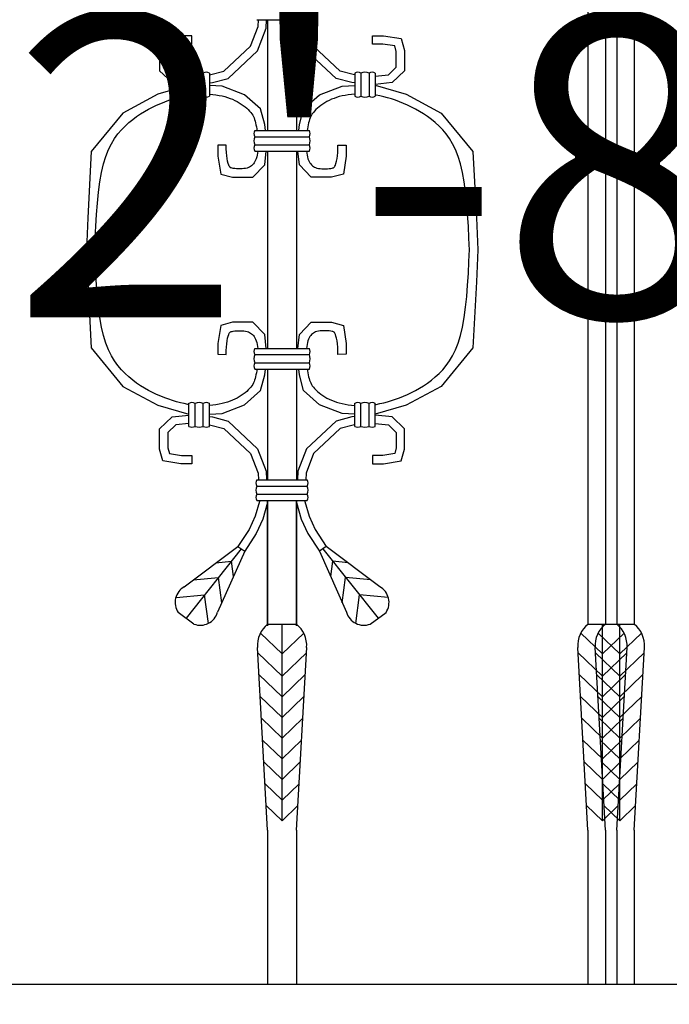
# Model space of a CAD drawing. Units: inches. Extents: x 2278 to 7495, y -71 to 1198.
# Tile 28 of 44: x 5114.19 to 5127.04, y 126.41 to 145.88. Entities that reach past the tile are written whole.
import ezdxf

# ---------------------------------------------------------------- set-up
doc = ezdxf.new("R2010")
doc.units = ezdxf.units.IN
doc.header["$MEASUREMENT"] = 0
doc.layers.add('A-ANNO-DIMS', color=2, linetype='Continuous', lineweight=18)
doc.layers.add('A-ELEV', color=7, linetype='Continuous', lineweight=25)
doc.styles.get("Standard").update_dxf_attribs({"font": 'arial.ttf'})
doc.dimstyles.get("Standard").update_dxf_attribs({"dimtxt": 6, "dimasz": 3, "dimexe": 0.18, "dimexo": 0.0625, "dimgap": 0.09, "dimtad": 0, "dimtih": 1, "dimtoh": 1, "dimdec": 0, "dimzin": 0, "dimdsep": 46, "dimlunit": 3, "dimtxsty": 'Standard', "dimblk": 'ARCHTICK', "dimcen": 0.09, "dimadec": 0, "dimazin": 0, "dimtfac": 1, "dimtdec": 0, "dimtofl": 0, "dimtmove": 0, "dimatfit": 3, "dimfxl": 1, "dimtolj": 1, "dimtzin": 0, "dimarcsym": 0})

# ---------------------------------------------------------------- blocks, each defined once
blk = doc.blocks.new('BALUSTER-ORNATE-B')
for p, q in [((3.37, 19.077), (4.37, 19.077)), ((3.396, 18.942), (3.402, 19.077)), ((3.558, 18.908), (3.565, 19.077)), ((3.585, 19.077), (3.585, 16.887)), ((4.155, 19.077), (4.155, 16.887)), ((4.183, 18.908), (4.175, 19.077)), ((4.344, 18.942), (4.338, 19.077)), ((3.247, 18.557), (3.396, 18.942)), ((3.386, 18.463), (3.558, 18.908)), ((4.355, 18.463), (4.183, 18.908)), ((4.494, 18.557), (4.344, 18.942)), ((1.513, 18.705), (1.449, 18.469)), ((1.867, 18.759), (1.513, 18.705)), ((2.084, 18.759), (1.867, 18.759)), ((2.084, 18.596), (2.084, 18.759)), ((5.656, 18.596), (5.656, 18.759)), ((5.656, 18.759), (5.874, 18.759)), ((5.874, 18.759), (6.228, 18.705)), ((6.228, 18.705), (6.291, 18.469)), ((1.612, 18.447), (1.643, 18.56)), ((1.643, 18.56), (1.879, 18.596)), ((1.879, 18.596), (2.084, 18.596)), ((2.72, 18.062), (3.247, 18.557)), ((5.021, 18.062), (4.494, 18.557)), ((5.861, 18.596), (5.656, 18.596)), ((6.098, 18.56), (5.861, 18.596)), ((6.128, 18.447), (6.098, 18.56)), ((1.449, 18.469), (1.449, 18.069)), ((1.612, 18.138), (1.612, 18.447)), ((2.801, 17.915), (3.386, 18.463)), ((4.939, 17.915), (4.355, 18.463)), ((6.128, 18.138), (6.128, 18.447)), ((6.291, 18.469), (6.291, 18.069)), ((1.767, 17.989), (1.612, 18.138)), ((5.973, 17.989), (6.128, 18.138)), ((1.449, 18.069), (1.694, 17.833)), ((2.027, 17.961), (1.767, 17.989)), ((2.027, 18.021), (2.027, 17.565)), ((2.149, 18.021), (2.149, 17.565)), ((2.312, 18.021), (2.312, 17.565)), ((2.434, 18.021), (2.434, 17.565)), ((2.434, 17.99), (2.462, 17.993)), ((2.462, 17.993), (2.72, 18.062)), ((2.493, 17.833), (2.801, 17.915)), ((5.248, 17.833), (4.939, 17.915)), ((5.279, 17.993), (5.021, 18.062)), ((5.307, 17.99), (5.279, 17.993)), ((5.307, 18.021), (5.307, 17.565)), ((5.429, 18.021), (5.429, 17.565)), ((5.592, 18.021), (5.592, 17.565)), ((5.714, 18.021), (5.714, 17.565)), ((5.714, 17.961), (5.973, 17.989)), ((6.291, 18.069), (6.046, 17.833)), ((2.027, 17.782), (1.412, 17.603)), ((1.694, 17.833), (2.027, 17.797)), ((2.434, 17.826), (2.493, 17.833)), ((2.684, 17.766), (2.434, 17.777)), ((3.128, 17.594), (2.684, 17.766)), ((4.612, 17.594), (5.057, 17.766)), ((5.057, 17.766), (5.307, 17.777)), ((5.307, 17.826), (5.248, 17.833)), ((6.046, 17.833), (5.714, 17.797)), ((5.714, 17.782), (6.328, 17.603)), ((1.412, 17.603), (0.722, 17.231)), ((1.705, 17.51), (1.782, 17.533)), ((1.782, 17.533), (1.858, 17.553)), ((1.858, 17.553), (1.933, 17.571)), ((1.933, 17.571), (2.008, 17.585)), ((2.008, 17.585), (2.027, 17.587)), ((2.434, 17.606), (2.5, 17.6)), ((2.5, 17.6), (2.563, 17.592)), ((2.563, 17.592), (2.625, 17.582)), ((2.625, 17.582), (2.683, 17.57)), ((2.683, 17.57), (2.739, 17.556)), ((2.739, 17.556), (2.792, 17.54)), ((2.792, 17.54), (2.843, 17.522)), ((2.843, 17.522), (2.891, 17.503)), ((3.446, 17.313), (3.128, 17.594)), ((4.294, 17.313), (4.612, 17.594)), ((4.898, 17.522), (4.849, 17.503)), ((4.948, 17.54), (4.898, 17.522)), ((5.002, 17.556), (4.948, 17.54)), ((5.057, 17.57), (5.002, 17.556)), ((5.116, 17.582), (5.057, 17.57)), ((5.177, 17.592), (5.116, 17.582)), ((5.241, 17.6), (5.177, 17.592)), ((5.307, 17.606), (5.241, 17.6)), ((5.733, 17.585), (5.714, 17.587)), ((5.807, 17.571), (5.733, 17.585)), ((5.882, 17.553), (5.807, 17.571)), ((5.958, 17.533), (5.882, 17.553)), ((6.035, 17.51), (5.958, 17.533)), ((6.328, 17.603), (7.018, 17.231)), ((1.23, 17.309), (1.309, 17.35)), ((1.309, 17.35), (1.389, 17.388)), ((1.389, 17.388), (1.469, 17.422)), ((1.469, 17.422), (1.549, 17.454)), ((1.549, 17.454), (1.628, 17.484)), ((1.628, 17.484), (1.705, 17.51)), ((2.891, 17.503), (2.937, 17.482)), ((2.937, 17.482), (2.982, 17.46)), ((2.982, 17.46), (3.024, 17.436)), ((3.024, 17.436), (3.064, 17.41)), ((3.064, 17.41), (3.103, 17.384)), ((3.103, 17.384), (3.138, 17.357)), ((3.138, 17.357), (3.171, 17.329)), ((3.171, 17.329), (3.201, 17.301)), ((4.569, 17.329), (4.539, 17.301)), ((4.602, 17.357), (4.569, 17.329)), ((4.638, 17.384), (4.602, 17.357)), ((4.676, 17.41), (4.638, 17.384)), ((4.717, 17.436), (4.676, 17.41)), ((4.759, 17.46), (4.717, 17.436)), ((4.803, 17.482), (4.759, 17.46)), ((4.849, 17.503), (4.803, 17.482)), ((6.113, 17.484), (6.035, 17.51)), ((6.192, 17.454), (6.113, 17.484)), ((6.271, 17.422), (6.192, 17.454)), ((6.351, 17.388), (6.271, 17.422)), ((6.431, 17.35), (6.351, 17.388)), ((6.511, 17.309), (6.431, 17.35)), ((0.722, 17.231), (0.096, 16.469)), ((0.916, 17.105), (0.994, 17.163)), ((0.994, 17.163), (1.072, 17.216)), ((1.072, 17.216), (1.151, 17.265)), ((1.151, 17.265), (1.23, 17.309)), ((3.201, 17.301), (3.228, 17.272)), ((3.228, 17.272), (3.252, 17.244)), ((3.252, 17.244), (3.272, 17.217)), ((3.272, 17.217), (3.289, 17.19)), ((3.289, 17.19), (3.303, 17.162)), ((3.303, 17.162), (3.316, 17.134)), ((3.316, 17.134), (3.327, 17.104)), ((3.528, 17.004), (3.446, 17.313)), ((4.213, 17.004), (4.294, 17.313)), ((4.425, 17.134), (4.413, 17.104)), ((4.437, 17.162), (4.425, 17.134)), ((4.452, 17.19), (4.437, 17.162)), ((4.469, 17.217), (4.452, 17.19)), ((4.489, 17.244), (4.469, 17.217)), ((4.512, 17.272), (4.489, 17.244)), ((4.539, 17.301), (4.512, 17.272)), ((6.59, 17.265), (6.511, 17.309)), ((6.669, 17.216), (6.59, 17.265)), ((6.747, 17.163), (6.669, 17.216)), ((6.825, 17.105), (6.747, 17.163)), ((7.018, 17.231), (7.645, 16.469)), ((0.692, 16.9), (0.765, 16.975)), ((0.765, 16.975), (0.839, 17.043)), ((0.839, 17.043), (0.916, 17.105)), ((3.327, 17.104), (3.337, 17.072)), ((3.337, 17.072), (3.346, 17.038)), ((3.346, 17.038), (3.354, 17.001)), ((3.354, 17.001), (3.362, 16.962)), ((3.362, 16.962), (3.369, 16.922)), ((3.542, 16.887), (3.528, 17.004)), ((4.199, 16.887), (4.213, 17.004)), ((4.379, 16.962), (4.372, 16.922)), ((4.387, 17.001), (4.379, 16.962)), ((4.395, 17.038), (4.387, 17.001)), ((4.404, 17.072), (4.395, 17.038)), ((4.413, 17.104), (4.404, 17.072)), ((6.901, 17.043), (6.825, 17.105)), ((6.976, 16.975), (6.901, 17.043)), ((7.048, 16.9), (6.976, 16.975)), ((0.557, 16.727), (0.623, 16.819)), ((0.623, 16.819), (0.692, 16.9)), ((3.33, 16.887), (4.411, 16.887)), ((3.33, 16.764), (4.411, 16.764)), ((3.369, 16.922), (3.374, 16.887)), ((4.372, 16.922), (4.366, 16.887)), ((7.117, 16.819), (7.048, 16.9)), ((7.183, 16.727), (7.117, 16.819)), ((0.438, 16.508), (0.496, 16.624)), ((0.496, 16.624), (0.557, 16.727)), ((2.765, 16.599), (2.602, 16.596)), ((2.602, 16.596), (2.602, 16.378)), ((2.766, 16.522), (2.765, 16.599)), ((3.33, 16.601), (4.411, 16.601)), ((4.975, 16.522), (4.976, 16.599)), ((4.976, 16.599), (5.139, 16.596)), ((5.139, 16.596), (5.139, 16.378)), ((7.245, 16.624), (7.183, 16.727)), ((7.302, 16.508), (7.245, 16.624)), ((0.096, 16.469), (0.025, 15.162)), ((0.34, 16.227), (0.386, 16.376)), ((0.386, 16.376), (0.438, 16.508)), ((2.602, 16.378), (2.656, 16.024)), ((2.769, 16.452), (2.766, 16.522)), ((2.775, 16.388), (2.769, 16.452)), ((2.783, 16.331), (2.775, 16.388)), ((3.33, 16.479), (4.411, 16.479)), ((3.368, 16.364), (3.358, 16.329)), ((3.377, 16.401), (3.368, 16.364)), ((3.384, 16.441), (3.377, 16.401)), ((3.388, 16.479), (3.384, 16.441)), ((3.528, 16.206), (3.558, 16.479)), ((3.585, 16.479), (3.585, 12.578)), ((4.155, 16.479), (4.155, 12.578)), ((4.213, 16.206), (4.183, 16.479)), ((4.352, 16.479), (4.357, 16.441)), ((4.357, 16.441), (4.364, 16.401)), ((4.364, 16.401), (4.373, 16.364)), ((4.373, 16.364), (4.383, 16.329)), ((4.958, 16.331), (4.965, 16.388)), ((4.965, 16.388), (4.971, 16.452)), ((4.971, 16.452), (4.975, 16.522)), ((5.139, 16.378), (5.084, 16.024)), ((7.354, 16.376), (7.302, 16.508)), ((7.401, 16.227), (7.354, 16.376)), ((7.645, 16.469), (7.715, 15.162)), ((0.3, 16.057), (0.34, 16.227)), ((2.793, 16.28), (2.783, 16.331)), ((2.803, 16.237), (2.793, 16.28)), ((2.815, 16.203), (2.803, 16.237)), ((2.826, 16.18), (2.815, 16.203)), ((2.834, 16.166), (2.826, 16.18)), ((2.841, 16.159), (2.834, 16.166)), ((2.846, 16.154), (2.841, 16.159)), ((3.229, 16.164), (3.206, 16.154)), ((3.249, 16.176), (3.229, 16.164)), ((3.269, 16.19), (3.249, 16.176)), ((3.286, 16.207), (3.269, 16.19)), ((3.303, 16.225), (3.286, 16.207)), ((3.292, 15.961), (3.528, 16.206)), ((3.319, 16.247), (3.303, 16.225)), ((3.333, 16.271), (3.319, 16.247)), ((3.346, 16.299), (3.333, 16.271)), ((3.358, 16.329), (3.346, 16.299)), ((4.449, 15.961), (4.213, 16.206)), ((4.383, 16.329), (4.394, 16.299)), ((4.394, 16.299), (4.407, 16.271)), ((4.407, 16.271), (4.422, 16.247)), ((4.422, 16.247), (4.437, 16.225)), ((4.437, 16.225), (4.454, 16.207)), ((4.454, 16.207), (4.472, 16.19)), ((4.472, 16.19), (4.491, 16.176)), ((4.491, 16.176), (4.512, 16.164)), ((4.512, 16.164), (4.535, 16.154)), ((4.895, 16.154), (4.9, 16.159)), ((4.9, 16.159), (4.906, 16.166)), ((4.906, 16.166), (4.915, 16.18)), ((4.915, 16.18), (4.926, 16.203)), ((4.926, 16.203), (4.937, 16.237)), ((4.937, 16.237), (4.948, 16.28)), ((4.948, 16.28), (4.958, 16.331)), ((7.44, 16.057), (7.401, 16.227)), ((0.267, 15.87), (0.3, 16.057)), ((2.656, 16.024), (2.892, 15.961)), ((2.852, 16.151), (2.846, 16.154)), ((2.863, 16.146), (2.852, 16.151)), ((2.881, 16.142), (2.863, 16.146)), ((2.905, 16.137), (2.881, 16.142)), ((2.936, 16.134), (2.905, 16.137)), ((2.971, 16.131), (2.936, 16.134)), ((3.008, 16.129), (2.971, 16.131)), ((3.045, 16.129), (3.008, 16.129)), ((3.082, 16.13), (3.045, 16.129)), ((3.117, 16.133), (3.082, 16.13)), ((3.15, 16.138), (3.117, 16.133)), ((3.18, 16.145), (3.15, 16.138)), ((3.206, 16.154), (3.18, 16.145)), ((4.535, 16.154), (4.561, 16.145)), ((4.561, 16.145), (4.591, 16.138)), ((4.591, 16.138), (4.624, 16.133)), ((4.624, 16.133), (4.659, 16.13)), ((4.659, 16.13), (4.696, 16.129)), ((4.696, 16.129), (4.733, 16.129)), ((4.733, 16.129), (4.769, 16.131)), ((4.769, 16.131), (4.805, 16.134)), ((4.805, 16.134), (4.836, 16.137)), ((4.836, 16.137), (4.86, 16.142)), ((5.084, 16.024), (4.848, 15.961)), ((4.86, 16.142), (4.877, 16.146)), ((4.877, 16.146), (4.888, 16.151)), ((4.888, 16.151), (4.895, 16.154)), ((7.473, 15.87), (7.44, 16.057)), ((0.24, 15.667), (0.267, 15.87)), ((2.892, 15.961), (3.292, 15.961)), ((4.848, 15.961), (4.449, 15.961)), ((7.501, 15.667), (7.473, 15.87)), ((0.217, 15.452), (0.24, 15.667)), ((7.523, 15.452), (7.501, 15.667)), ((0.199, 15.227), (0.217, 15.452)), ((7.541, 15.227), (7.523, 15.452)), ((0.185, 14.995), (0.199, 15.227)), ((7.556, 14.995), (7.541, 15.227)), ((0.025, 15.162), (0, 14.529)), ((0.173, 14.759), (0.185, 14.995)), ((7.567, 14.759), (7.556, 14.995)), ((7.715, 15.162), (7.74, 14.529)), ((0.163, 14.522), (0.173, 14.759)), ((7.577, 14.522), (7.567, 14.759)), ((0, 14.529), (0.025, 13.895)), ((0.173, 14.298), (0.163, 14.536)), ((7.567, 14.298), (7.577, 14.536)), ((7.74, 14.529), (7.715, 13.895)), ((0.185, 14.062), (0.173, 14.298)), ((7.556, 14.062), (7.567, 14.298)), ((0.199, 13.831), (0.185, 14.062)), ((7.541, 13.831), (7.556, 14.062)), ((0.025, 13.895), (0.096, 12.589)), ((0.217, 13.606), (0.199, 13.831)), ((7.523, 13.606), (7.541, 13.831)), ((7.715, 13.895), (7.645, 12.589)), ((0.24, 13.391), (0.217, 13.606)), ((7.501, 13.391), (7.523, 13.606)), ((0.267, 13.188), (0.24, 13.391)), ((7.473, 13.188), (7.501, 13.391)), ((0.3, 13), (0.267, 13.188)), ((2.892, 13.097), (2.656, 13.033)), ((3.292, 13.097), (2.892, 13.097)), ((3.528, 12.852), (3.292, 13.097)), ((4.213, 12.852), (4.449, 13.097)), ((4.449, 13.097), (4.848, 13.097)), ((4.848, 13.097), (5.084, 13.033)), ((7.44, 13), (7.473, 13.188)), ((0.34, 12.831), (0.3, 13)), ((2.656, 13.033), (2.602, 12.679)), ((2.803, 12.82), (2.815, 12.854)), ((2.815, 12.854), (2.826, 12.878)), ((2.826, 12.878), (2.834, 12.892)), ((2.834, 12.892), (2.841, 12.899)), ((2.841, 12.899), (2.846, 12.903)), ((2.846, 12.903), (2.852, 12.907)), ((2.852, 12.907), (2.863, 12.911)), ((2.863, 12.911), (2.881, 12.916)), ((2.881, 12.916), (2.905, 12.92)), ((2.905, 12.92), (2.936, 12.924)), ((2.936, 12.924), (2.971, 12.927)), ((2.971, 12.927), (3.008, 12.929)), ((3.008, 12.929), (3.045, 12.929)), ((3.045, 12.929), (3.082, 12.928)), ((3.082, 12.928), (3.117, 12.924)), ((3.117, 12.924), (3.15, 12.919)), ((3.15, 12.919), (3.18, 12.912)), ((3.18, 12.912), (3.206, 12.904)), ((3.206, 12.904), (3.229, 12.893)), ((3.229, 12.893), (3.249, 12.881)), ((3.249, 12.881), (3.269, 12.867)), ((3.269, 12.867), (3.286, 12.851)), ((3.286, 12.851), (3.303, 12.832)), ((3.558, 12.578), (3.528, 12.852)), ((4.183, 12.578), (4.213, 12.852)), ((4.454, 12.851), (4.437, 12.832)), ((4.472, 12.867), (4.454, 12.851)), ((4.491, 12.881), (4.472, 12.867)), ((4.512, 12.893), (4.491, 12.881)), ((4.535, 12.904), (4.512, 12.893)), ((4.561, 12.912), (4.535, 12.904)), ((4.591, 12.919), (4.561, 12.912)), ((4.624, 12.924), (4.591, 12.919)), ((4.659, 12.928), (4.624, 12.924)), ((4.696, 12.929), (4.659, 12.928)), ((4.733, 12.929), (4.696, 12.929)), ((4.769, 12.927), (4.733, 12.929)), ((4.805, 12.924), (4.769, 12.927)), ((4.836, 12.92), (4.805, 12.924)), ((4.86, 12.916), (4.836, 12.92)), ((4.877, 12.911), (4.86, 12.916)), ((4.888, 12.907), (4.877, 12.911)), ((4.895, 12.903), (4.888, 12.907)), ((4.9, 12.899), (4.895, 12.903)), ((4.906, 12.892), (4.9, 12.899)), ((4.915, 12.878), (4.906, 12.892)), ((4.926, 12.854), (4.915, 12.878)), ((4.937, 12.82), (4.926, 12.854)), ((5.084, 13.033), (5.139, 12.679)), ((7.401, 12.831), (7.44, 13)), ((0.386, 12.681), (0.34, 12.831)), ((0.438, 12.549), (0.386, 12.681)), ((2.602, 12.679), (2.602, 12.462)), ((2.769, 12.605), (2.775, 12.669)), ((2.775, 12.669), (2.783, 12.727)), ((2.783, 12.727), (2.793, 12.778)), ((2.793, 12.778), (2.803, 12.82)), ((3.303, 12.832), (3.319, 12.811)), ((3.319, 12.811), (3.333, 12.786)), ((3.333, 12.786), (3.346, 12.759)), ((3.346, 12.759), (3.358, 12.728)), ((3.358, 12.728), (3.368, 12.694)), ((3.368, 12.694), (3.377, 12.656)), ((3.377, 12.656), (3.384, 12.616)), ((4.364, 12.656), (4.357, 12.616)), ((4.373, 12.694), (4.364, 12.656)), ((4.383, 12.728), (4.373, 12.694)), ((4.394, 12.759), (4.383, 12.728)), ((4.407, 12.786), (4.394, 12.759)), ((4.422, 12.811), (4.407, 12.786)), ((4.437, 12.832), (4.422, 12.811)), ((4.948, 12.778), (4.937, 12.82)), ((4.958, 12.727), (4.948, 12.778)), ((4.965, 12.669), (4.958, 12.727)), ((4.971, 12.605), (4.965, 12.669)), ((5.139, 12.679), (5.139, 12.462)), ((7.302, 12.549), (7.354, 12.681)), ((7.354, 12.681), (7.401, 12.831)), ((0.096, 12.589), (0.722, 11.827)), ((0.496, 12.433), (0.438, 12.549)), ((2.602, 12.462), (2.765, 12.459)), ((2.765, 12.459), (2.766, 12.536)), ((2.766, 12.536), (2.769, 12.605)), ((3.33, 12.578), (4.411, 12.578)), ((3.384, 12.616), (3.388, 12.578)), ((4.357, 12.616), (4.352, 12.578)), ((4.975, 12.536), (4.971, 12.605)), ((4.976, 12.459), (4.975, 12.536)), ((5.139, 12.462), (4.976, 12.459)), ((7.645, 12.589), (7.018, 11.827)), ((7.245, 12.433), (7.302, 12.549)), ((0.557, 12.33), (0.496, 12.433)), ((0.623, 12.239), (0.557, 12.33)), ((3.33, 12.456), (4.411, 12.456)), ((3.33, 12.293), (4.411, 12.293)), ((7.117, 12.239), (7.183, 12.33)), ((7.183, 12.33), (7.245, 12.433)), ((0.692, 12.157), (0.623, 12.239)), ((0.765, 12.083), (0.692, 12.157)), ((0.839, 12.015), (0.765, 12.083)), ((3.33, 12.171), (4.411, 12.171)), ((3.362, 12.095), (3.354, 12.056)), ((3.369, 12.136), (3.362, 12.095)), ((3.374, 12.171), (3.369, 12.136)), ((3.528, 12.053), (3.542, 12.171)), ((3.585, 12.171), (3.585, 9.98)), ((4.155, 12.171), (4.155, 9.98)), ((4.213, 12.053), (4.199, 12.171)), ((4.366, 12.171), (4.372, 12.136)), ((4.372, 12.136), (4.379, 12.095)), ((4.379, 12.095), (4.387, 12.056)), ((6.901, 12.015), (6.976, 12.083)), ((6.976, 12.083), (7.048, 12.157)), ((7.048, 12.157), (7.117, 12.239)), ((0.916, 11.952), (0.839, 12.015)), ((0.994, 11.894), (0.916, 11.952)), ((1.072, 11.841), (0.994, 11.894)), ((3.303, 11.895), (3.289, 11.868)), ((3.316, 11.924), (3.303, 11.895)), ((3.327, 11.954), (3.316, 11.924)), ((3.337, 11.986), (3.327, 11.954)), ((3.346, 12.02), (3.337, 11.986)), ((3.354, 12.056), (3.346, 12.02)), ((3.446, 11.745), (3.528, 12.053)), ((4.294, 11.745), (4.213, 12.053)), ((4.387, 12.056), (4.395, 12.02)), ((4.395, 12.02), (4.404, 11.986)), ((4.404, 11.986), (4.413, 11.954)), ((4.413, 11.954), (4.425, 11.924)), ((4.425, 11.924), (4.437, 11.895)), ((4.437, 11.895), (4.452, 11.868)), ((6.669, 11.841), (6.747, 11.894)), ((6.747, 11.894), (6.825, 11.952)), ((6.825, 11.952), (6.901, 12.015)), ((0.722, 11.827), (1.412, 11.455)), ((1.151, 11.793), (1.072, 11.841)), ((1.23, 11.748), (1.151, 11.793)), ((1.309, 11.708), (1.23, 11.748)), ((1.389, 11.67), (1.309, 11.708)), ((3.138, 11.701), (3.103, 11.673)), ((3.128, 11.464), (3.446, 11.745)), ((3.171, 11.729), (3.138, 11.701)), ((3.201, 11.757), (3.171, 11.729)), ((3.228, 11.785), (3.201, 11.757)), ((3.252, 11.813), (3.228, 11.785)), ((3.272, 11.841), (3.252, 11.813)), ((3.289, 11.868), (3.272, 11.841)), ((4.612, 11.464), (4.294, 11.745)), ((4.452, 11.868), (4.469, 11.841)), ((4.469, 11.841), (4.489, 11.813)), ((4.489, 11.813), (4.512, 11.785)), ((4.512, 11.785), (4.539, 11.757)), ((4.539, 11.757), (4.569, 11.729)), ((4.569, 11.729), (4.602, 11.701)), ((4.602, 11.701), (4.638, 11.673)), ((7.018, 11.827), (6.328, 11.455)), ((6.351, 11.67), (6.431, 11.708)), ((6.431, 11.708), (6.511, 11.748)), ((6.511, 11.748), (6.59, 11.793)), ((6.59, 11.793), (6.669, 11.841)), ((1.469, 11.635), (1.389, 11.67)), ((1.549, 11.603), (1.469, 11.635)), ((1.628, 11.574), (1.549, 11.603)), ((1.705, 11.548), (1.628, 11.574)), ((1.782, 11.524), (1.705, 11.548)), ((1.858, 11.504), (1.782, 11.524)), ((1.933, 11.487), (1.858, 11.504)), ((2.008, 11.473), (1.933, 11.487)), ((2.027, 11.037), (2.027, 11.493)), ((2.149, 11.037), (2.149, 11.493)), ((2.312, 11.037), (2.312, 11.493)), ((2.434, 11.037), (2.434, 11.493)), ((2.683, 11.488), (2.625, 11.476)), ((2.739, 11.502), (2.683, 11.488)), ((2.792, 11.518), (2.739, 11.502)), ((2.843, 11.535), (2.792, 11.518)), ((2.891, 11.555), (2.843, 11.535)), ((2.937, 11.576), (2.891, 11.555)), ((2.982, 11.598), (2.937, 11.576)), ((3.024, 11.622), (2.982, 11.598)), ((3.064, 11.647), (3.024, 11.622)), ((3.103, 11.673), (3.064, 11.647)), ((4.638, 11.673), (4.676, 11.647)), ((4.676, 11.647), (4.717, 11.622)), ((4.717, 11.622), (4.759, 11.598)), ((4.759, 11.598), (4.803, 11.576)), ((4.803, 11.576), (4.849, 11.555)), ((4.849, 11.555), (4.898, 11.535)), ((4.898, 11.535), (4.948, 11.518)), ((4.948, 11.518), (5.002, 11.502)), ((5.002, 11.502), (5.057, 11.488)), ((5.057, 11.488), (5.116, 11.476)), ((5.307, 11.037), (5.307, 11.493)), ((5.429, 11.037), (5.429, 11.493)), ((5.592, 11.037), (5.592, 11.493)), ((5.714, 11.037), (5.714, 11.493)), ((5.733, 11.473), (5.807, 11.487)), ((5.807, 11.487), (5.882, 11.504)), ((5.882, 11.504), (5.958, 11.524)), ((5.958, 11.524), (6.035, 11.548)), ((6.035, 11.548), (6.113, 11.574)), ((6.113, 11.574), (6.192, 11.603)), ((6.192, 11.603), (6.271, 11.635)), ((6.271, 11.635), (6.351, 11.67)), ((1.412, 11.455), (2.027, 11.276)), ((2.027, 11.47), (2.008, 11.473)), ((2.5, 11.457), (2.434, 11.451)), ((2.434, 11.28), (2.684, 11.291)), ((2.563, 11.465), (2.5, 11.457)), ((2.625, 11.476), (2.563, 11.465)), ((2.684, 11.291), (3.128, 11.464)), ((5.057, 11.291), (4.612, 11.464)), ((5.307, 11.28), (5.057, 11.291)), ((5.116, 11.476), (5.177, 11.465)), ((5.177, 11.465), (5.241, 11.457)), ((5.241, 11.457), (5.307, 11.451)), ((5.714, 11.47), (5.733, 11.473)), ((6.328, 11.455), (5.714, 11.276)), ((1.449, 10.988), (1.694, 11.225)), ((1.694, 11.225), (2.027, 11.261)), ((2.027, 11.097), (1.767, 11.069)), ((2.434, 11.232), (2.493, 11.225)), ((2.493, 11.225), (2.801, 11.143)), ((2.801, 11.143), (3.386, 10.594)), ((4.939, 11.143), (4.355, 10.594)), ((5.248, 11.225), (4.939, 11.143)), ((5.307, 11.232), (5.248, 11.225)), ((6.046, 11.225), (5.714, 11.261)), ((5.714, 11.097), (5.973, 11.069)), ((6.291, 10.988), (6.046, 11.225)), ((1.449, 10.589), (1.449, 10.988)), ((1.767, 11.069), (1.612, 10.919)), ((1.612, 10.919), (1.612, 10.611)), ((2.434, 11.067), (2.462, 11.064)), ((2.462, 11.064), (2.72, 10.996)), ((2.72, 10.996), (3.247, 10.501)), ((5.021, 10.996), (4.494, 10.501)), ((5.279, 11.064), (5.021, 10.996)), ((5.307, 11.067), (5.279, 11.064)), ((5.973, 11.069), (6.128, 10.919)), ((6.128, 10.919), (6.128, 10.611)), ((6.291, 10.589), (6.291, 10.988)), ((1.513, 10.353), (1.449, 10.589)), ((1.612, 10.611), (1.643, 10.498)), ((3.386, 10.594), (3.558, 10.149)), ((4.355, 10.594), (4.183, 10.149)), ((6.128, 10.611), (6.098, 10.498)), ((6.228, 10.353), (6.291, 10.589)), ((1.867, 10.298), (1.513, 10.353)), ((1.643, 10.498), (1.879, 10.461)), ((1.879, 10.461), (2.084, 10.461)), ((2.084, 10.461), (2.084, 10.298)), ((3.247, 10.501), (3.396, 10.115)), ((4.494, 10.501), (4.344, 10.115)), ((5.861, 10.461), (5.656, 10.461)), ((5.656, 10.461), (5.656, 10.298)), ((6.098, 10.498), (5.861, 10.461)), ((5.874, 10.298), (6.228, 10.353)), ((2.084, 10.298), (1.867, 10.298)), ((3.558, 10.149), (3.565, 9.98)), ((4.183, 10.149), (4.175, 9.98)), ((5.656, 10.298), (5.874, 10.298)), ((3.37, 9.98), (4.37, 9.98)), ((3.396, 10.115), (3.402, 9.98)), ((4.344, 10.115), (4.338, 9.98)), ((3.37, 9.858), (4.37, 9.858)), ((3.421, 9.552), (3.337, 9.262)), ((3.37, 9.695), (4.37, 9.695)), ((3.37, 9.573), (4.37, 9.573)), ((3.42, 9.573), (3.421, 9.552)), ((3.583, 9.573), (3.585, 9.532)), ((3.585, 9.573), (3.585, 7.095)), ((3.585, 7.095), (3.585, 9.573)), ((4.155, 9.573), (4.155, 7.095)), ((4.155, 7.095), (4.155, 9.573)), ((4.157, 9.573), (4.155, 9.532)), ((4.32, 9.573), (4.319, 9.552)), ((4.319, 9.552), (4.404, 9.262)), ((3.585, 9.532), (3.49, 9.205)), ((4.155, 9.532), (4.251, 9.205)), ((3.337, 9.262), (3.217, 9.001)), ((3.49, 9.205), (3.36, 8.922)), ((4.251, 9.205), (4.381, 8.922)), ((4.404, 9.262), (4.524, 9.001)), ((3.217, 9.001), (2.995, 8.66)), ((4.524, 9.001), (4.746, 8.66)), ((3.36, 8.922), (3.132, 8.571)), ((4.381, 8.922), (4.609, 8.571)), ((1.936, 7.866), (2.995, 8.66)), ((3.063, 8.615), (1.971, 7.244)), ((3.132, 8.571), (2.595, 7.362)), ((2.995, 8.66), (3.132, 8.571)), ((4.746, 8.66), (4.609, 8.571)), ((4.609, 8.571), (5.146, 7.362)), ((4.677, 8.615), (5.77, 7.244)), ((5.804, 7.866), (4.746, 8.66)), ((2.563, 8.34), (2.868, 8.37)), ((2.907, 8.066), (2.868, 8.37)), ((4.833, 8.066), (4.873, 8.37)), ((5.178, 8.34), (4.873, 8.37)), ((2.112, 8.002), (2.614, 8.051)), ((2.679, 7.551), (2.614, 8.051)), ((5.062, 7.551), (5.127, 8.051)), ((5.629, 8.002), (5.127, 8.051)), ((1.774, 7.651), (2.339, 7.706)), ((2.412, 7.143), (2.339, 7.706)), ((5.328, 7.143), (5.402, 7.706)), ((5.966, 7.651), (5.402, 7.706)), ((2.128, 7.128), (1.814, 7.359)), ((5.613, 7.128), (5.927, 7.359)), ((3.585, 7.128), (4.155, 7.128)), ((3.87, 3.24), (3.87, 7.128)), ((3.442, 6.952), (3.87, 6.538)), ((4.299, 6.952), (3.87, 6.538)), ((3.585, 3.055), (3.383, 6.664)), ((4.155, 3.055), (4.358, 6.664)), ((3.389, 6.562), (3.87, 6.097)), ((4.352, 6.562), (3.87, 6.097)), ((3.413, 6.131), (3.87, 5.689)), ((4.328, 6.131), (3.87, 5.689)), ((3.437, 5.699), (3.87, 5.28)), ((4.304, 5.699), (3.87, 5.28)), ((3.461, 5.268), (3.87, 4.872)), ((4.279, 5.268), (3.87, 4.872)), ((3.485, 4.836), (3.87, 4.464)), ((4.255, 4.836), (3.87, 4.464)), ((3.51, 4.405), (3.87, 4.056)), ((4.231, 4.405), (3.87, 4.056)), ((3.534, 3.973), (3.87, 3.648)), ((4.207, 3.973), (3.87, 3.648)), ((3.558, 3.542), (3.87, 3.24)), ((4.183, 3.542), (3.87, 3.24)), ((3.585, 3.055), (3.585, 0)), ((4.155, 3.055), (4.155, 0))]:
    blk.add_line(p, q)
for centre, radius, start, end in [((2.088, 17.916), 0.121, 59.7768, 120.2232), ((2.23, 17.828), 0.209, 67.1017, 112.8983), ((2.373, 17.916), 0.121, 59.7768, 120.2232), ((5.368, 17.916), 0.121, 59.7768, 120.2232), ((5.51, 17.828), 0.209, 67.1017, 112.8983), ((5.653, 17.916), 0.121, 59.7768, 120.2232), ((2.088, 17.67), 0.121, 239.7768, 300.2232), ((2.23, 17.758), 0.209, 247.1017, 292.8983), ((2.373, 17.67), 0.121, 239.7768, 300.2232), ((5.368, 17.67), 0.121, 239.7768, 300.2232), ((5.51, 17.758), 0.209, 247.1017, 292.8983), ((5.653, 17.67), 0.121, 239.7768, 300.2232), ((3.434, 16.825), 0.121, 149.7768, 210.2232), ((3.522, 16.683), 0.209, 157.1017, 202.8983), ((4.306, 16.825), 0.121, 329.7768, 30.2232), ((4.218, 16.683), 0.209, 337.1017, 22.8983), ((3.434, 16.54), 0.121, 149.7768, 210.2232), ((4.306, 16.54), 0.121, 329.7768, 30.2232), ((3.434, 12.517), 0.121, 149.7768, 210.2232), ((4.306, 12.517), 0.121, 329.7768, 30.2232), ((3.522, 12.375), 0.209, 157.1017, 202.8983), ((3.434, 12.232), 0.121, 149.7768, 210.2232), ((4.218, 12.375), 0.209, 337.1017, 22.8983), ((4.306, 12.232), 0.121, 329.7768, 30.2232), ((2.088, 11.388), 0.121, 59.7768, 120.2232), ((2.23, 11.3), 0.209, 67.1017, 112.8983), ((2.373, 11.388), 0.121, 59.7768, 120.2232), ((5.368, 11.388), 0.121, 59.7768, 120.2232), ((5.51, 11.3), 0.209, 67.1017, 112.8983), ((5.653, 11.388), 0.121, 59.7768, 120.2232), ((2.088, 11.142), 0.121, 239.7768, 300.2232), ((2.23, 11.23), 0.209, 247.1017, 292.8983), ((2.373, 11.142), 0.121, 239.7768, 300.2232), ((5.368, 11.142), 0.121, 239.7768, 300.2232), ((5.51, 11.23), 0.209, 247.1017, 292.8983), ((5.653, 11.142), 0.121, 239.7768, 300.2232), ((3.475, 9.919), 0.121, 149.7768, 210.2232), ((4.265, 9.919), 0.121, 329.7768, 30.2232), ((3.563, 9.776), 0.209, 157.1017, 202.8983), ((4.177, 9.776), 0.209, 337.1017, 22.8983), ((3.475, 9.634), 0.121, 149.7768, 210.2232), ((4.265, 9.634), 0.121, 329.7768, 30.2232), ((2.111, 7.555), 0.356, 119.3212, 213.425), ((5.63, 7.555), 0.356, 326.575, 60.6788), ((2.253, 7.462), 0.356, 249.4937, 343.5975), ((5.488, 7.462), 0.356, 196.4025, 290.5063), ((3.929, 6.703), 0.547, 128.9283, 183.9822), ((3.811, 6.703), 0.547, 356.0178, 51.0717)]:
    blk.add_arc(centre, radius, start, end)
blk = doc.blocks.new('_ArchTick')
at = {"color": 0, "linetype": 'ByBlock', "const_width": 0.15}
blk.add_lwpolyline([(-0.5, -0.5), (0.5, 0.5)], dxfattribs=at)
blk = doc.blocks.new('*D59')
at = {"layer": 'A-ANNO-DIMS', "color": 0, "lineweight": -2, "transparency": 16777216}
for p, q in [((5096.589, 159.183), (5101.564, 159.183)), ((5101.384, 159.183), (5101.384, 146.185)), ((5101.384, 126.799), (5101.384, 139.796)), ((5096.589, 126.799), (5101.564, 126.799))]:
    blk.add_line(p, q, dxfattribs=at)
at = {"layer": 'Defpoints', "color": 0, "transparency": 16777216}
for p in [(5096.527, 159.183), (5101.384, 159.183), (5096.527, 126.799)]:
    blk.add_point(p, dxfattribs=at)
at = {"layer": 'A-ANNO-DIMS', "color": 0, "lineweight": -2, "transparency": 16777216, "xscale": 3, "yscale": 3, "zscale": 3}
for p, rotation in [((5101.384, 159.183), 90), ((5101.384, 126.799), 270)]:
    blk.add_blockref('_ArchTick', p, dxfattribs=dict(at, rotation=rotation))
at = {"layer": 'A-ANNO-DIMS', "color": 0, "transparency": 16777216, "insert": (5101.384, 142.991), "char_height": 6, "attachment_point": 5}
blk.add_mtext('\\A1;ORNATE BALUSTER 2\'-8 1/2" TYP.', dxfattribs=at)
blk = doc.blocks.new('*D60')
at = {"layer": 'A-ANNO-DIMS', "color": 0, "lineweight": -2, "transparency": 16777216}
for p, q in [((5088.787, 126.736), (5088.787, 121.761)), ((5096.527, 126.736), (5096.527, 121.761)), ((5088.787, 121.941), (5096.527, 121.941)), ((5096.527, 121.941), (5099.527, 121.941))]:
    blk.add_line(p, q, dxfattribs=at)
at = {"layer": 'Defpoints', "color": 0, "transparency": 16777216}
for p in [(5088.787, 126.799), (5096.527, 126.799), (5096.527, 121.941)]:
    blk.add_point(p, dxfattribs=at)
at = {"layer": 'A-ANNO-DIMS', "color": 0, "lineweight": -2, "transparency": 16777216, "xscale": 3, "yscale": 3, "zscale": 3, "rotation": 180}
blk.add_blockref('_ArchTick', (5088.787, 121.941), dxfattribs=at)
at = {"layer": 'A-ANNO-DIMS', "color": 0, "lineweight": -2, "transparency": 16777216, "xscale": 3, "yscale": 3, "zscale": 3}
blk.add_blockref('_ArchTick', (5096.527, 121.941), dxfattribs=at)
at = {"layer": 'A-ANNO-DIMS', "color": 0, "transparency": 16777216, "insert": (5124.894, 121.941), "char_height": 6, "attachment_point": 5}
blk.add_mtext('\\A1;0\'-7 1/2" TYP.', dxfattribs=at)
blk = doc.blocks.new('*D123')
at = {"layer": 'A-ANNO-DIMS', "color": 0, "lineweight": -2, "transparency": 16777216}
for p, q in [((4736.95, 340.157), (4736.95, -23.427)), ((5145.676, -1.81), (5145.676, -23.427)), ((4736.95, -23.247), (4923.929, -23.247)), ((5145.676, -23.247), (4958.697, -23.247))]:
    blk.add_line(p, q, dxfattribs=at)
at = {"layer": 'Defpoints', "color": 0, "transparency": 16777216}
for p in [(4736.95, 340.219), (5145.676, -1.747), (5145.676, -23.247)]:
    blk.add_point(p, dxfattribs=at)
at = {"layer": 'A-ANNO-DIMS', "color": 0, "lineweight": -2, "transparency": 16777216, "xscale": 3, "yscale": 3, "zscale": 3, "rotation": 180}
blk.add_blockref('_ArchTick', (4736.95, -23.247), dxfattribs=at)
at = {"layer": 'A-ANNO-DIMS', "color": 0, "lineweight": -2, "transparency": 16777216, "xscale": 3, "yscale": 3, "zscale": 3}
blk.add_blockref('_ArchTick', (5145.676, -23.247), dxfattribs=at)
at = {"layer": 'A-ANNO-DIMS', "color": 0, "transparency": 16777216, "insert": (4941.313, -23.247), "char_height": 6, "attachment_point": 5}
blk.add_mtext('\\A1;34\'-0 1/2"', dxfattribs=at)
blk = doc.blocks.new('*D131')
at = {"layer": 'A-ANNO-DIMS', "color": 0, "lineweight": -2, "transparency": 16777216}
for p, q in [((5096.176, 99.315), (5096.176, 361.899)), ((5145.676, 118.315), (5145.676, 361.899)), ((5096.176, 361.719), (5105.75, 361.719)), ((5145.676, 361.719), (5136.102, 361.719))]:
    blk.add_line(p, q, dxfattribs=at)
at = {"layer": 'Defpoints', "color": 0, "transparency": 16777216}
for p in [(5145.676, 361.719), (5145.676, 118.253), (5096.176, 99.253)]:
    blk.add_point(p, dxfattribs=at)
at = {"layer": 'A-ANNO-DIMS', "color": 0, "lineweight": -2, "transparency": 16777216, "xscale": 3, "yscale": 3, "zscale": 3, "rotation": 180}
blk.add_blockref('_ArchTick', (5096.176, 361.719), dxfattribs=at)
at = {"layer": 'A-ANNO-DIMS', "color": 0, "lineweight": -2, "transparency": 16777216, "xscale": 3, "yscale": 3, "zscale": 3}
blk.add_blockref('_ArchTick', (5145.676, 361.719), dxfattribs=at)
at = {"layer": 'A-ANNO-DIMS', "color": 0, "transparency": 16777216, "insert": (5120.926, 361.719), "char_height": 6, "attachment_point": 5}
blk.add_mtext('\\A1;4\'-1 1/2"', dxfattribs=at)
blk = doc.blocks.new('*D139')
at = {"layer": 'A-ANNO-DIMS', "color": 0, "lineweight": -2, "transparency": 16777216}
for p, q in [((5092.239, 160.253), (5167.754, 160.253)), ((5167.574, 160.253), (5167.574, 142.408)), ((5167.574, 118.253), (5167.574, 136.097)), ((5145.739, 118.253), (5167.754, 118.253))]:
    blk.add_line(p, q, dxfattribs=at)
at = {"layer": 'Defpoints', "color": 0, "transparency": 16777216}
for p in [(5092.176, 160.253), (5167.574, 160.253), (5145.676, 118.253)]:
    blk.add_point(p, dxfattribs=at)
at = {"layer": 'A-ANNO-DIMS', "color": 0, "lineweight": -2, "transparency": 16777216, "xscale": 3, "yscale": 3, "zscale": 3}
for p, rotation in [((5167.574, 160.253), 90), ((5167.574, 118.253), 270)]:
    blk.add_blockref('_ArchTick', p, dxfattribs=dict(at, rotation=rotation))
at = {"layer": 'A-ANNO-DIMS', "color": 0, "transparency": 16777216, "insert": (5167.574, 139.253), "char_height": 6, "attachment_point": 5}
blk.add_mtext('\\A1;3\'-6"', dxfattribs=at)

msp = doc.modelspace()

# ---------------------------------------------------------------- linework, layer by layer
at = {"layer": 'A-ELEV'}
for p, q in [((5125.431, 148.728), (5125.431, 133.927)), ((5125.775, 148.728), (5125.775, 133.927)), ((5126.001, 148.728), (5126.001, 133.927)), ((5126.345, 148.728), (5126.345, 133.927)), ((5125.431, 133.927), (5126.001, 133.927)), ((5125.716, 130.039), (5125.716, 133.927)), ((5125.775, 133.927), (5126.345, 133.927)), ((5126.06, 130.039), (5126.06, 133.927)), ((5125.287, 133.751), (5125.716, 133.337)), ((5125.631, 133.751), (5126.06, 133.337)), ((5126.144, 133.751), (5125.716, 133.337)), ((5126.488, 133.751), (5126.06, 133.337)), ((5125.431, 129.854), (5125.229, 133.463)), ((5125.234, 133.361), (5125.716, 132.896)), ((5125.775, 129.854), (5125.573, 133.463)), ((5125.578, 133.361), (5126.06, 132.896)), ((5126.198, 133.361), (5125.716, 132.896)), ((5126.001, 129.854), (5126.203, 133.463)), ((5126.541, 133.361), (5126.06, 132.896)), ((5126.345, 129.854), (5126.547, 133.463)), ((5125.259, 132.93), (5125.716, 132.488)), ((5125.602, 132.93), (5126.06, 132.488)), ((5126.173, 132.93), (5125.716, 132.488)), ((5126.517, 132.93), (5126.06, 132.488)), ((5125.283, 132.498), (5125.716, 132.079)), ((5125.627, 132.498), (5126.06, 132.079)), ((5126.149, 132.498), (5125.716, 132.079)), ((5126.493, 132.498), (5126.06, 132.079)), ((5125.307, 132.067), (5125.716, 131.671)), ((5125.651, 132.067), (5126.06, 131.671)), ((5126.125, 132.067), (5125.716, 131.671)), ((5126.469, 132.067), (5126.06, 131.671)), ((5125.331, 131.635), (5125.716, 131.263)), ((5125.675, 131.635), (5126.06, 131.263)), ((5126.101, 131.635), (5125.716, 131.263)), ((5126.445, 131.635), (5126.06, 131.263)), ((5125.355, 131.204), (5125.716, 130.855)), ((5125.699, 131.204), (5126.06, 130.855)), ((5126.077, 131.204), (5125.716, 130.855)), ((5126.421, 131.204), (5126.06, 130.855)), ((5125.379, 130.772), (5125.716, 130.447)), ((5126.053, 130.772), (5125.716, 130.447)), ((5125.723, 130.772), (5126.06, 130.447)), ((5126.396, 130.772), (5126.06, 130.447)), ((5125.404, 130.341), (5125.716, 130.039)), ((5126.028, 130.341), (5125.716, 130.039)), ((5125.747, 130.341), (5126.06, 130.039)), ((5126.372, 130.341), (5126.06, 130.039)), ((5125.431, 129.854), (5125.431, 126.799)), ((5125.775, 129.854), (5125.775, 126.799)), ((5126.001, 129.854), (5126.001, 126.799)), ((5126.345, 129.854), (5126.345, 126.799)), ((5145.676, 126.799), (5066.016, 126.799))]:
    msp.add_line(p, q, dxfattribs=at)
for centre, start, end in [((5125.775, 133.502), 128.9283, 183.9822), ((5126.119, 133.502), 128.9283, 183.9822), ((5125.657, 133.502), 356.0178, 51.0717), ((5126.001, 133.502), 356.0178, 51.0717)]:
    msp.add_arc(centre, 0.547, start, end, dxfattribs=at)

# ---------------------------------------------------------------- block references
msp.add_blockref('BALUSTER-ORNATE-B', (5115.509, 126.799), dxfattribs=at)

# ---------------------------------------------------------------- dimensions: what is measured, and where the dimension line sits
at = {"layer": 'A-ANNO-DIMS'}
for base, p1, p2, picture, middle in [((5145.676, 361.719), (5096.176, 99.253), (5145.676, 118.253), '*D131', (5120.926, 361.719)), ((5145.676, -23.247), (4736.95, 340.219), (5145.676, -1.747), '*D123', (4941.313, -23.247))]:
    dim = msp.add_linear_dim(base=base, p1=p1, p2=p2, dimstyle='Standard', override={"dimdec": 1, "dimlfac": 1, "dimrnd": 0, "dimzin": 1, "dimdsep": 46, "dimlunit": 4, "dimfrac": 2}, dxfattribs=at)
    dim.commit()
    dim.dimension.update_dxf_attribs({"geometry": picture, "text_midpoint": middle})
dim = msp.add_linear_dim(base=(5101.384, 159.183), p1=(5096.527, 126.799), p2=(5096.527, 159.183), angle=90, text='ORNATE BALUSTER <> TYP.', dimstyle='Standard', override={"dimdec": 1, "dimrnd": 0, "dimzin": 1, "dimlunit": 4, "dimfrac": 2}, dxfattribs=at)
dim.commit()
dim.dimension.update_dxf_attribs({"geometry": '*D59', "text_midpoint": (5101.384, 142.991)})
dim = msp.add_linear_dim(base=(5167.574, 160.253), p1=(5145.676, 118.253), p2=(5092.176, 160.253), angle=90, dimstyle='Standard', override={"dimdec": 1, "dimlfac": 1, "dimrnd": 0, "dimzin": 1, "dimdsep": 46, "dimlunit": 4, "dimfrac": 2}, dxfattribs=at)
dim.commit()
dim.dimension.update_dxf_attribs({"geometry": '*D139', "text_midpoint": (5167.574, 139.253)})
dim = msp.add_linear_dim(base=(5096.527, 121.941), p1=(5088.787, 126.799), p2=(5096.527, 126.799), text='<> TYP.', dimstyle='Standard', override={"dimdec": 1, "dimrnd": 0, "dimzin": 1, "dimlunit": 4, "dimfrac": 2}, dxfattribs=at)
dim.commit()
dim.dimension.update_dxf_attribs({"geometry": '*D60', "text_midpoint": (5124.894, 121.941)})

doc.saveas('drawing.dxf')
